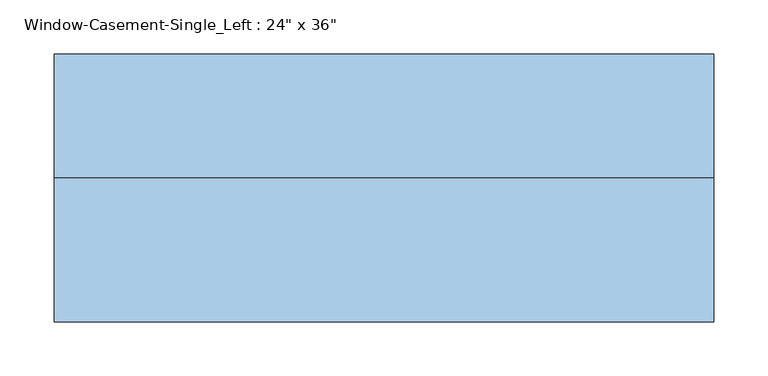
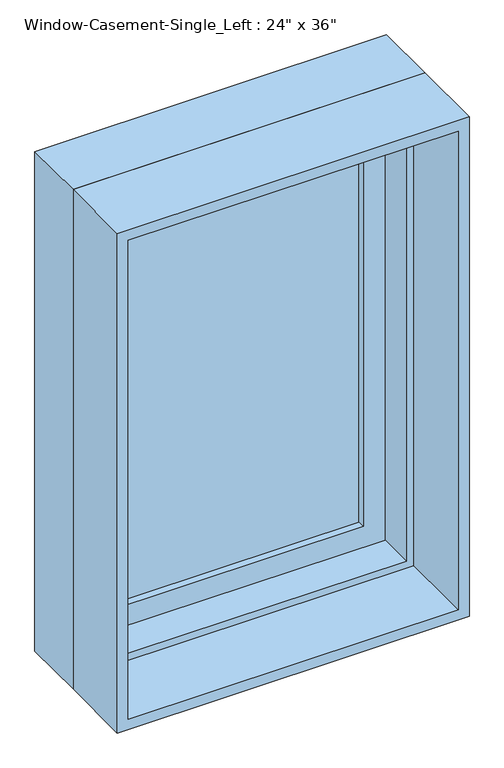
"""IFC4 building model written with IfcOpenShell, lengths in millimetres: window geometry."""

from ifc_helpers import new_model, si_unit, frame, origin, place, context, project, spatial, polyline, outline, extrude, faceted_brep, source, transform, mapped, element, save


def window_bab9308a(model_context):
    return source(origin(), model_context, "Body", "SolidModel", [
        faceted_brep([(273.05, 82.55, 1797.05), (273.05, 19.05, 1797.05), (-273.05, 19.05, 1797.05), (-273.05, 82.55, 1797.05), (292.1, 133.35, 1816.1), (292.1, 82.55, 1816.1), (-292.1, 82.55, 1816.1), (-292.1, 133.35, 1816.1), (304.8, 19.05, 1828.8), (304.8, 133.35, 1828.8), (-304.8, 133.35, 1828.8), (-304.8, 19.05, 1828.8), (-273.05, 19.05, 946.15), (-273.05, 82.55, 946.15), (-292.1, 82.55, 927.1), (-292.1, 133.35, 927.1), (-304.8, 133.35, 914.4), (-304.8, 19.05, 914.4), (273.05, 19.05, 946.15), (273.05, 82.55, 946.15), (292.1, 82.55, 927.1), (292.1, 133.35, 927.1), (304.8, 133.35, 914.4), (304.8, 19.05, 914.4)], [[[0, 1, 2, 3]], [[4, 5, 6, 7]], [[8, 9, 10, 11]], [[3, 2, 12, 13]], [[7, 6, 14, 15]], [[11, 10, 16, 17]], [[13, 12, 18, 19]], [[15, 14, 20, 21]], [[17, 16, 22, 23]], [[11, 17, 23, 8], [1, 18, 12, 2]], [[19, 18, 1, 0]], [[5, 20, 14, 6], [3, 13, 19, 0]], [[21, 20, 5, 4]], [[23, 22, 9, 8]], [[9, 22, 16, 10], [7, 15, 21, 4]]]),
        extrude(outline(polyline([(1828.8, -304.8), (914.4, -304.8), (914.4, 304.8), (1828.8, 304.8), (1828.8, -304.8)]), holes=[polyline([(1809.75, 285.75), (933.45, 285.75), (933.45, -285.75), (1809.75, -285.75), (1809.75, 285.75)])]), frame((0.0, -114.3, 0.0), z_axis=(0.0, 1.0, 0.0), x_axis=(0.0, 0.0, 1.0)), (0.0, 0.0, 1.0), 133.35),
        extrude(outline(polyline([(1816.1, -292.1), (927.1, -292.1), (927.1, 292.1), (1816.1, 292.1), (1816.1, -292.1)]), holes=[polyline([(1758.95, 234.95), (984.25, 234.95), (984.25, -234.95), (1758.95, -234.95), (1758.95, 234.95)])]), frame((0.0, 82.55, 0.0), z_axis=(0.0, 1.0, 0.0), x_axis=(0.0, 0.0, 1.0)), (0.0, 0.0, 1.0), 44.45),
        extrude(outline(polyline([(234.95, 114.3), (234.95, 107.95), (-234.95, 107.95), (-234.95, 114.3), (234.95, 114.3)])), frame((0.0, 0.0, 984.25), z_axis=(0.0, 0.0, 1.0), x_axis=(1.0, 0.0, 0.0)), (0.0, 0.0, 1.0), 774.7),
        extrude(outline(polyline([(-234.95, 95.25), (-234.95, 101.6), (234.95, 101.6), (234.95, 95.25), (-234.95, 95.25)])), frame((0.0, 0.0, 984.25), z_axis=(0.0, 0.0, 1.0), x_axis=(1.0, 0.0, 0.0)), (0.0, 0.0, 1.0), 774.7),
    ])


if __name__ == "__main__":
    model = new_model("IFC4")
    model_context = context("Model", 3, world=origin())
    ifc_project = project(units=[si_unit("LENGTHUNIT", "METRE", prefix="MILLI")], contexts=[model_context])
    site = spatial("IfcSite", under=ifc_project)
    building = spatial("IfcBuilding", under=site)
    placement = place(None, origin())
    window_shape = window_bab9308a(model_context)
    element("IfcWindow", 1, ObjectType="Window-Casement-Single_Left : 24\" x 36\"", at=placement, inside=building, context=model_context, shape_type="MappedRepresentation", body=[
        mapped(window_shape, transform((0.0, 0.0, 0.0), x_axis=(1.0, 0.0, 0.0), y_axis=(0.0, 1.0, 0.0), z_axis=(0.0, 0.0, 1.0))),
    ])
    save(model, "model.ifc")

# Revit data of these elements
# Type "Window-Casement-Single_Left : 24\" x 36\""
#   Type Mark = "18"
#   Fire Rating = "0.5h"
#   Assembly Code = "B2020100"
#   Analytic Construction = "Double glazing - domestic"
#   Window Inset [instance default] = 0' - 0"
#   Wall Thickness [instance default] = 0' - 6"
#   Visual Light Transmittance = 0.81
#   Thermal Resistance (R) = 1.8146 (h·ft²·°F)/BTU
#   Solar Heat Gain Coefficient = 0.76
#   Rough Width = 2' - 0 1/2"
#   Rough Height = 3' - 0 1/2"
#   Interior Wall Closure [instance default] = 0' - 2 1/4"
#   Height = 3' - 0"
#   Heat Transfer Coefficient (U) = 0.5511 BTU/(h·ft²·°F)
#   Frame Extension [instance default] = 0' - 0 1/4"
#   Exterior Wall Closure [instance default] = 0' - 1 1/4"
#   Extension Jamb [instance default] = 0' - 2 1/4"
#   Default Sill Height = 3' - 0"
#   Width = 2' - 0"
#   Muntin Visibility = yes
#   Interior Trim Visibility [instance default] = yes
#   Exterior Trim Visibility [instance default] = yes
#   Extension Jamb Visibility [instance default] = yes
#   Muntin Pattern = Muntin Pattern_2x2 : Muntin Pattern_2x2
#   Interior Trim Material = Wood - Stained
#   Interior Trim = Trim-Window-Interior-Flat : Picture Frame
#   Interior Frame Material = Wood - Stained
#   Glass Panel Material = Glass
#   Exterior Trim Material = Clad - White
#   Exterior Trim = Trim-Window-Exterior-Flat : with Sill
#   Exterior Frame Material = Clad - White
#   Wall Closure = (empty or 0)
# Element 1 (IfcWindow, "Window-Casement-Single_Left : 24\" x 36\"")
#   Wall Thickness = 0' - 9"
#   Extension Jamb = 0' - 5 1/4"
#   Materials on its faces: "Wood - Stained", "Glass", "Clad - White"
# Materials
#   "Wood - Stained": class "Wood", colour RGB 224 178 126, transparency 0, Cost = 0
#   "Glass": class "Glass", colour RGB 0 128 192, transparency 0.75, Description = "Soda Lime Glass", Cost = 0
#   "Clad - White": class "Wood", colour RGB 242 242 238, transparency 0, Cost = 0
